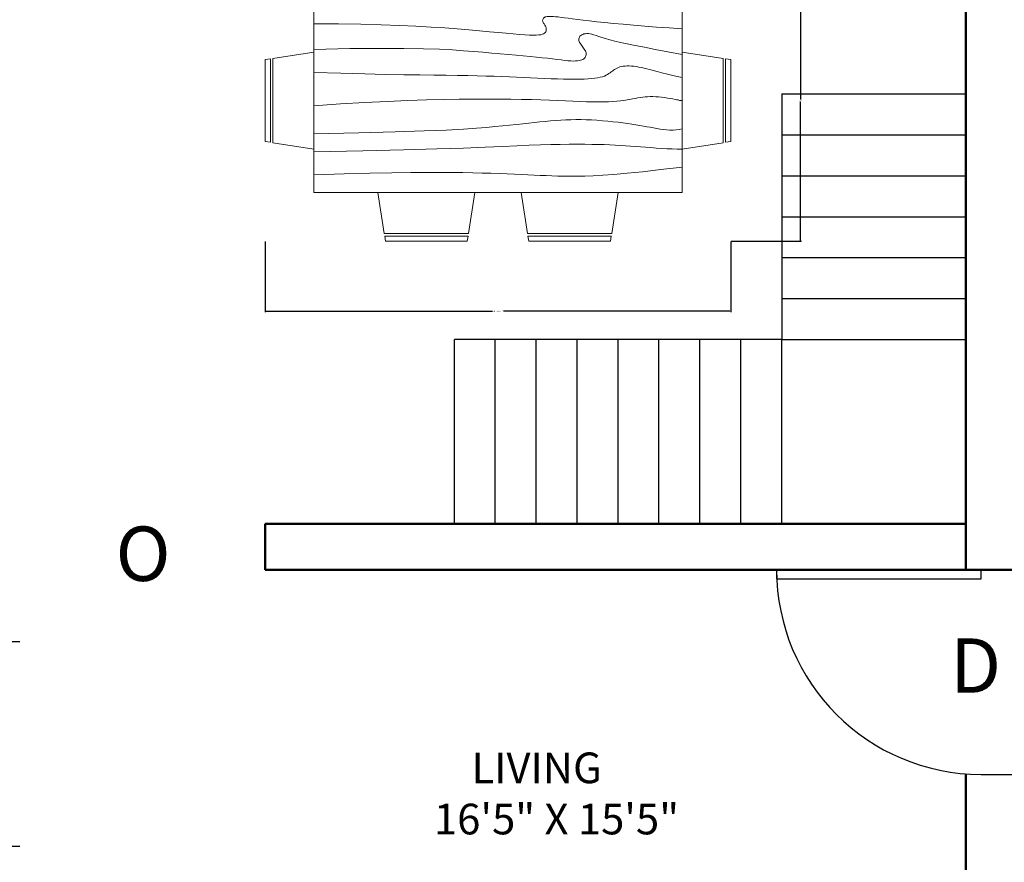
# Model space of a CAD drawing. Units: inches. Extents: x -105 to 1196, y -792 to 119.
# Tile 17 of 23: x 130 to 322, y -285 to -121. Entities that reach past the tile are written whole.
import ezdxf

# ---------------------------------------------------------------- set-up
doc = ezdxf.new("R2010")
doc.units = ezdxf.units.IN
doc.header["$MEASUREMENT"] = 0
for name, color, linetype, lineweight in [('A-ANNO-DIMS', 2, 'Continuous', 18), ('A-ANNO-TEXT', 7, 'Continuous', 25), ('A-AREA-IDEN', 7, 'Continuous', 25), ('A-DOOR', 4, 'Continuous', 25), ('A-FLOR-STRS', 4, 'Continuous', 25), ('A-FURN', 8, 'Continuous', 18), ('A-WALL', 3, 'Continuous', 50)]:
    doc.layers.add(name, color=color, linetype=linetype, lineweight=lineweight)
doc.styles.get("Standard").update_dxf_attribs({"font": 'arial.ttf'})
doc.dimstyles.get("Standard").update_dxf_attribs({"dimtxt": 0.18, "dimasz": 0.18, "dimexe": 0.18, "dimexo": 0.0625, "dimgap": 0.09, "dimtad": 0, "dimtih": 1, "dimtoh": 1, "dimdec": 1, "dimzin": 0, "dimdsep": 46, "dimlunit": 4, "dimtxsty": 'Standard', "dimcen": 0.09, "dimadec": 0, "dimazin": 0, "dimtfac": 1, "dimtdec": 1, "dimtofl": 0, "dimtmove": 0, "dimatfit": 3, "dimfxl": 1, "dimtolj": 1, "dimtzin": 0, "dimarcsym": 0})

# ---------------------------------------------------------------- blocks, each defined once
blk = doc.blocks.new('Dining Set - 36 x 72 in.')
for p, q in [((-22, 27.5), (-22.1562, 26.50042)), ((-22, 27.5), (-6, 27.5)), ((-5.8437, 26.49966), (-6, 27.5)), ((6, 27.5), (5.8438, 26.50042)), ((6, 27.5), (22, 27.5)), ((22.1563, 26.49966), (22, 27.5)), ((-22.2343, 26.00059), (-23.4847, 17.99762)), ((-22.2304, 26), (-5.7608, 26)), ((-5.8416, 26.5), (-22.1534, 26.5)), ((-4.5152, 17.99762), (-5.7655, 25.99926)), ((5.7657, 26.00059), (4.5153, 17.99762)), ((5.7696, 26), (22.2392, 26)), ((22.1584, 26.5), (5.8466, 26.5)), ((23.4848, 17.99762), (22.2345, 25.99926)), ((36, 18), (-36, 18)), ((-36, 18), (-36, -18)), ((36, -18), (36, 18)), ((-45.5, 8), (-44.5004, 8.15617)), ((-45.5, 8), (-45.5, -8)), ((-44.5, -8.15843), (-44.5, 8.15338)), ((-44.0006, 8.23428), (-35.9976, 9.48474)), ((-44, 8.23041), (-44, -8.23915)), ((44.0006, 8.23428), (35.9976, 9.48474)), ((44, 8.23041), (44, -8.23915)), ((44.5, -8.15843), (44.5, 8.15338)), ((45.5, 8), (44.5005, 8.15617)), ((45.5, 8), (45.5, -8)), ((-44.4997, -8.15631), (-45.5, -8)), ((-35.9976, -9.48476), (-43.9993, -8.2345)), ((35.9976, -9.48476), (43.9993, -8.2345)), ((44.4997, -8.15631), (45.5, -8)), ((-36, -18), (36, -18)), ((-22.2343, -26.0006), (-23.4847, -17.99762)), ((-4.5152, -17.99762), (-5.7655, -25.99928)), ((5.7657, -26.0006), (4.5153, -17.99762)), ((23.4848, -17.99762), (22.2345, -25.99928)), ((-22.2304, -26), (-5.7608, -26)), ((-22, -27.5), (-22.1562, -26.50044)), ((-5.8416, -26.5), (-22.1534, -26.5)), ((-5.8437, -26.49967), (-6, -27.5)), ((5.7696, -26), (22.2392, -26)), ((6, -27.5), (5.8438, -26.50044)), ((22.1584, -26.5), (5.8466, -26.5)), ((22.1563, -26.49967), (22, -27.5)), ((-22, -27.5), (-6, -27.5)), ((6, -27.5), (22, -27.5))]:
    blk.add_line(p, q)
for points in [[(-36, 15), (-31.1772, 14.97754), (-26.8079, 14.91406), (-22.8538, 14.81543), (-19.276, 14.6875), (-16.0362, 14.53613), (-13.0957, 14.36718), (-10.4159, 14.18652), (-7.9583, 14), (-5.6904, 13.81315), (-3.6035, 13.63021), (-1.6954, 13.45508), (0.0365, 13.29166), (1.5945, 13.14388), (2.9811, 13.01562), (4.1988, 12.9108), (5.25, 12.83333), (6.1393, 12.78613), (6.8802, 12.76823), (7.4883, 12.77767), (7.9792, 12.8125), (8.3685, 12.87077), (8.6719, 12.95052), (8.9049, 13.0498), (9.0833, 13.16666), (9.2205, 13.29899), (9.3216, 13.44401), (9.3895, 13.59879), (9.4271, 13.76041), (9.4373, 13.92594), (9.4232, 14.09245), (9.3875, 14.257), (9.3333, 14.41666), (9.2638, 14.56917), (9.1836, 14.71484), (9.0975, 14.85465), (9.0104, 14.98958), (8.9272, 15.1206), (8.8529, 15.2487), (8.7922, 15.37483), (8.75, 15.5), (8.7305, 15.62467), (8.7344, 15.74739), (8.7617, 15.86621), (8.8125, 15.97916), (8.8867, 16.08431), (8.9844, 16.17968), (9.1055, 16.26334), (9.25, 16.33333), (9.4189, 16.38802), (9.6172, 16.42708), (9.8506, 16.45052), (10.125, 16.45833), (10.4463, 16.45052), (10.8203, 16.42708), (11.2529, 16.38802), (11.75, 16.33333), (12.3184, 16.26318), (12.9694, 16.17838), (13.7151, 16.07991), (14.5677, 15.96875), (15.5395, 15.84586), (16.6426, 15.71224), (17.8893, 15.56884), (19.2917, 15.41666), (20.859, 15.25667), (22.5879, 15.08984), (24.4721, 14.91715), (26.5052, 14.73958), (28.6809, 14.5581), (30.9929, 14.3737), (33.4347, 14.18733), (36, 14)], [(-36, 10), (-28.9766, 10.14274), (-23.1725, 10.20442), (-18.4241, 10.19775), (-14.5677, 10.13541), (-11.4399, 10.03011), (-8.877, 9.89453), (-6.7154, 9.74137), (-4.7917, 9.58333), (-2.9698, 9.43082), (-1.2246, 9.28515), (0.4415, 9.14534), (2.026, 9.01041), (3.5266, 8.87939), (4.9408, 8.7513), (6.266, 8.62516), (7.5, 8.5), (8.6411, 8.37549), (9.6914, 8.2539), (10.6538, 8.13818), (11.5312, 8.03125), (12.3267, 7.93603), (13.043, 7.85547), (13.6831, 7.79248), (14.25, 7.75), (14.7471, 7.7303), (15.1797, 7.73307), (15.5537, 7.75732), (15.875, 7.80208), (16.1494, 7.86637), (16.3828, 7.94922), (16.5811, 8.04964), (16.75, 8.16666), (16.8944, 8.29915), (17.0143, 8.44531), (17.1089, 8.60319), (17.1771, 8.77083), (17.218, 8.94629), (17.2305, 9.1276), (17.2137, 9.31282), (17.1667, 9.5), (17.0895, 9.6875), (16.987, 9.875), (16.8649, 10.0625), (16.7292, 10.25), (16.5856, 10.4375), (16.4401, 10.625), (16.2985, 10.8125), (16.1667, 11), (16.05, 11.18733), (15.9518, 11.3737), (15.8752, 11.5581), (15.8229, 11.73958), (15.798, 11.91715), (15.8034, 12.08984), (15.842, 12.25667), (15.9167, 12.41666), (16.0295, 12.56836), (16.1784, 12.70833), (16.3605, 12.83268), (16.5729, 12.9375), (16.8127, 13.01888), (17.0768, 13.07291), (17.3625, 13.0957), (17.6667, 13.08333), (17.9894, 13.03312), (18.3418, 12.94726), (18.7382, 12.82918), (19.1927, 12.68229), (19.7195, 12.51001), (20.3327, 12.31575), (21.0465, 12.10294), (21.875, 11.875), (22.8357, 11.63354), (23.959, 11.37304), (25.2786, 11.08618), (26.8282, 10.76562), (28.6414, 10.40405), (30.752, 9.99414), (33.1936, 9.52856), (36, 9)], [(-36, 5.5), (-30.7157, 5.3348), (-26.069, 5.20963), (-21.9946, 5.11767), (-18.4271, 5.05208), (-15.3009, 5.00602), (-12.5508, 4.97265), (-10.1112, 4.94515), (-7.9167, 4.91666), (-5.909, 4.88167), (-4.0586, 4.83984), (-2.3429, 4.79215), (-0.7396, 4.73958), (0.7739, 4.6831), (2.22, 4.6237), (3.6213, 4.56233), (5, 4.5), (6.373, 4.43782), (7.7344, 4.3776), (9.0723, 4.32129), (10.375, 4.27083), (11.6309, 4.22819), (12.8281, 4.19531), (13.9551, 4.17415), (15, 4.16666), (15.954, 4.17448), (16.819, 4.19791), (17.6001, 4.23698), (18.3021, 4.29166), (18.9299, 4.36198), (19.4883, 4.44791), (19.9823, 4.54948), (20.4167, 4.66666), (20.7969, 4.79899), (21.1302, 4.94401), (21.4245, 5.09879), (21.6875, 5.26041), (21.9271, 5.42594), (22.1511, 5.59245), (22.3672, 5.757), (22.5834, 5.91666), (22.8065, 6.06868), (23.0404, 6.21093), (23.2879, 6.34147), (23.5521, 6.45833), (23.8358, 6.55957), (24.142, 6.64323), (24.4735, 6.70735), (24.8334, 6.75), (25.2235, 6.76969), (25.642, 6.76692), (26.0858, 6.74267), (26.5521, 6.69791), (27.0379, 6.63362), (27.5404, 6.55078), (28.0565, 6.45036), (28.5834, 6.33333), (29.1242, 6.19987), (29.7071, 6.04687), (30.3661, 5.87044), (31.1354, 5.66666), (32.0493, 5.43164), (33.142, 5.16146), (34.4475, 4.85221), (36, 4.5)], [(-36, -1), (-30.7915, -0.6591), (-26.0195, -0.38216), (-21.6519, -0.16284), (-17.6563, 0.00521), (-14.0005, 0.12833), (-10.6523, 0.21289), (-7.5796, 0.26522), (-4.75, 0.29166), (-2.134, 0.29793), (0.2878, 0.28711), (2.5317, 0.26163), (4.6146, 0.22396), (6.5529, 0.17651), (8.3633, 0.12174), (10.0623, 0.06209), (11.6667, 0), (13.1899, -0.06201), (14.6341, -0.1211), (15.9982, -0.17432), (17.2813, -0.21875), (18.4823, -0.25147), (19.6003, -0.26953), (20.6343, -0.27002), (21.5834, -0.25), (22.4481, -0.20768), (23.2357, -0.14584), (23.9549, -0.06836), (24.6146, 0.02083), (25.2235, 0.11784), (25.7904, 0.21875), (26.3241, 0.31966), (26.8334, 0.41666), (27.3265, 0.50618), (27.8099, 0.58593), (28.2894, 0.65397), (28.7709, 0.70833), (29.2601, 0.74707), (29.763, 0.76823), (30.2855, 0.76985), (30.8334, 0.75), (31.4088, 0.70784), (31.9994, 0.64713), (32.589, 0.57275), (33.1615, 0.48958), (33.7008, 0.4025), (34.1908, 0.3164), (34.6153, 0.23616), (34.9584, 0.16666), (35.2099, 0.11165), (35.3848, 0.07031), (35.504, 0.04069), (35.5886, 0.02083), (35.6594, 0.00879), (35.7377, 0.0026), (35.8442, 0.00032), (36, 0)], [(-36, -6.5), (-27.1843, -6.31267), (-20.084, -6.1263), (-14.469, -5.9419), (-10.1094, -5.76042), (-6.7752, -5.58285), (-4.2363, -5.41016), (-2.2629, -5.24333), (-0.625, -5.08334), (0.8708, -4.93099), (2.2715, -4.78646), (3.5872, -4.64974), (4.8281, -4.52084), (6.0046, -4.39974), (7.127, -4.28646), (8.2053, -4.18099), (9.25, -4.08334), (10.2705, -3.99382), (11.2734, -3.91407), (12.2647, -3.84603), (13.25, -3.79167), (14.2354, -3.75293), (15.2266, -3.73177), (16.2295, -3.73015), (17.25, -3.75), (18.2912, -3.79248), (19.3451, -3.85547), (20.4009, -3.93604), (21.4479, -4.03125), (22.4754, -4.13819), (23.4727, -4.25391), (24.4289, -4.37549), (25.3334, -4.5), (26.1785, -4.62492), (26.9694, -4.74935), (27.7145, -4.87281), (28.4219, -4.99479), (29.1, -5.11483), (29.7572, -5.23242), (30.4016, -5.34709), (31.0417, -5.45834), (31.6837, -5.56437), (32.3262, -5.65821), (32.9658, -5.73153), (33.599, -5.77604), (34.2224, -5.78345), (34.8327, -5.74545), (35.4264, -5.65373), (36, -5.5)], [(-36, -10), (-26.4022, -9.81299), (-18.4675, -9.62891), (-11.9839, -9.45069), (-6.7396, -9.28125), (-2.5226, -9.12354), (0.8789, -8.98047), (3.6769, -8.85498), (6.0833, -8.75), (8.2767, -8.66765), (10.3021, -8.60677), (12.1712, -8.56543), (13.8958, -8.54167), (15.4876, -8.53353), (16.9583, -8.53907), (18.3197, -8.55632), (19.5834, -8.58334), (20.7616, -8.61841), (21.8685, -8.66081), (22.9188, -8.71004), (23.9271, -8.76563), (24.9081, -8.82707), (25.8763, -8.89388), (26.8465, -8.96558), (27.8334, -9.04167), (28.8474, -9.12118), (29.8828, -9.20117), (30.93, -9.27824), (31.9792, -9.34896), (33.0205, -9.40991), (34.0443, -9.45768), (35.0407, -9.48885), (36, -9.5)], [(-36, -14.5), (-30.0881, -14.33513), (-25.0332, -14.21224), (-20.7312, -14.12647), (-17.0781, -14.07292), (-13.97, -14.04671), (-11.3027, -14.04297), (-8.9724, -14.05681), (-6.875, -14.08334), (-4.9224, -14.11833), (-3.0905, -14.16016), (-1.3709, -14.20785), (0.2448, -14.26042), (1.7647, -14.3169), (3.1973, -14.3763), (4.5507, -14.43767), (5.8333, -14.5), (7.0554, -14.5621), (8.235, -14.62175), (9.3922, -14.67652), (10.5469, -14.72396), (11.7192, -14.76164), (12.929, -14.78711), (14.1965, -14.79794), (15.5417, -14.79167), (16.9933, -14.76424), (18.6152, -14.70508), (20.4804, -14.60197), (22.6615, -14.44271), (25.2312, -14.21509), (28.2624, -13.9069), (31.8277, -13.50594), (36, -13)]]:
    blk.add_lwpolyline(points)
blk = doc.blocks.new('*U24')
for p, q in [((0, 0), (0, -6)), ((-40, 0), (-40, -6))]:
    blk.add_line(p, q)
blk.add_lwpolyline([(0, 0), (0, 40), (-1.75, 40), (-1.75, 0)], close=True)
blk.add_arc((0, 0), 40, 90, 180)
blk = doc.blocks.new('*U4')
for p, q in [((0, 0), (0, -6)), ((40, 0), (40, -6))]:
    blk.add_line(p, q)
blk.add_lwpolyline([(0, 0), (0, 40), (1.75, 40), (1.75, 0)], close=True)
blk.add_arc((0, 0), 40, 0, 90)
blk = doc.blocks.new('*D75')
at = {"layer": 'A-ANNO-DIMS', "color": 0, "lineweight": -2, "transparency": 16777216}
for p, q in [((177.77, -164.1), (177.77, -177.86)), ((268.77, -164.1), (268.77, -177.86)), ((177.95, -177.68), (222.19, -177.68)), ((268.59, -177.68), (224.35, -177.68))]:
    blk.add_line(p, q, dxfattribs=at)
at = {"layer": 'A-ANNO-DIMS', "color": 0, "transparency": 16777216}
for points in [[(177.95, -177.65), (177.95, -177.71), (177.77, -177.68)], [(268.59, -177.65), (268.59, -177.71), (268.77, -177.68)]]:
    blk.add_solid(points, dxfattribs=at)
at = {"layer": 'Defpoints', "color": 0, "transparency": 16777216}
for p in [(177.77, -164.03), (268.77, -164.03), (268.77, -177.68)]:
    blk.add_point(p, dxfattribs=at)
at = {"layer": 'A-ANNO-DIMS', "color": 0, "transparency": 16777216, "insert": (223.27, -177.68), "char_height": 0.18, "attachment_point": 5}
blk.add_mtext('\\A1;DINING SET 7\'-7"', dxfattribs=at)
blk = doc.blocks.new('*D76')
at = {"layer": 'A-ANNO-DIMS', "color": 0, "lineweight": -2, "transparency": 16777216}
for p, q in [((268.83, -109.03), (282.6, -109.03)), ((282.42, -109.21), (282.42, -136.35)), ((282.42, -163.85), (282.42, -136.71)), ((268.83, -164.03), (282.6, -164.03))]:
    blk.add_line(p, q, dxfattribs=at)
at = {"layer": 'A-ANNO-DIMS', "color": 0, "transparency": 16777216}
for points in [[(282.39, -109.21), (282.45, -109.21), (282.42, -109.03)], [(282.39, -163.85), (282.45, -163.85), (282.42, -164.03)]]:
    blk.add_solid(points, dxfattribs=at)
at = {"layer": 'Defpoints', "color": 0, "transparency": 16777216}
for p in [(268.77, -109.03), (282.42, -109.03), (268.77, -164.03)]:
    blk.add_point(p, dxfattribs=at)
at = {"layer": 'A-ANNO-DIMS', "color": 0, "transparency": 16777216, "insert": (282.42, -136.53), "char_height": 0.18, "attachment_point": 5}
blk.add_mtext('\\A1;4\'-7"', dxfattribs=at)

msp = doc.modelspace()

# ---------------------------------------------------------------- linework, layer by layer
at = {"layer": 'A-FLOR-STRS'}
for p, q in [((278.74, -135.23), (314.74, -135.23)), ((278.74, -135.23), (278.74, -183.23)), ((278.74, -143.23), (314.74, -143.23)), ((278.74, -151.23), (314.74, -151.23)), ((278.74, -159.23), (314.74, -159.23)), ((278.74, -167.23), (314.74, -167.23)), ((278.74, -175.23), (314.74, -175.23)), ((214.74, -219.23), (214.74, -183.23)), ((278.74, -183.23), (214.74, -183.23)), ((222.74, -219.23), (222.74, -183.23)), ((230.74, -219.23), (230.74, -183.23)), ((238.74, -219.23), (238.74, -183.23)), ((246.74, -219.23), (246.74, -183.23)), ((254.74, -219.23), (254.74, -183.23)), ((262.74, -219.23), (262.74, -183.23)), ((270.74, -219.23), (270.74, -183.23)), ((278.74, -219.23), (278.74, -183.23)), ((278.74, -183.23), (314.74, -183.23))]:
    msp.add_line(p, q, dxfattribs=at)
at = {"layer": 'A-WALL'}
for p, q in [((314.74, -116.23), (314.74, -228.23)), ((314.74, -219.23), (177.74, -219.23)), ((177.74, -219.23), (177.74, -228.23)), ((323.74, -228.23), (177.74, -228.23)), ((314.74, -268.11), (314.74, -429.23))]:
    msp.add_line(p, q, dxfattribs=at)

# ---------------------------------------------------------------- block references
at = {"layer": 'A-DOOR', "rotation": 90}
for name, p in [('*U24', (317.74, -228.23)), ('*U4', (123.74, -282.23))]:
    msp.add_blockref(name, p, dxfattribs=at)
at = {"layer": 'A-FURN'}
msp.add_blockref('Dining Set - 36 x 72 in.', (223.27, -136.53), dxfattribs=at)

# ---------------------------------------------------------------- texts
at = {"layer": 'A-ANNO-TEXT'}
for s, p in [('O', (148.49, -230.42)), ('D', (311.66, -252.28))]:
    msp.add_text(s, height=10.64, dxfattribs=at).set_placement(p)
at = {"layer": 'A-AREA-IDEN', "insert": (210.74, -263.95), "char_height": 6, "attachment_point": 1}
msp.add_mtext_dynamic_manual_height_columns('    LIVING\\P16\'5" X 15\'5"', width=59.5623, gutter_width=1, heights=[0], dxfattribs=at)

# ---------------------------------------------------------------- dimensions: what is measured, and where the dimension line sits
at = {"layer": 'A-ANNO-DIMS'}
dim = msp.add_linear_dim(base=(282.42, -109.03), p1=(268.77, -164.03), p2=(268.77, -109.03), angle=90, dimstyle='Standard', override={"dimdec": 1, "dimlfac": 1, "dimrnd": 0, "dimzin": 1, "dimdsep": 46, "dimlunit": 4, "dimfrac": 2}, dxfattribs=at)
dim.commit()
dim.dimension.update_dxf_attribs({"geometry": '*D76', "text_midpoint": (282.42, -136.53)})
dim = msp.add_linear_dim(base=(268.77, -177.68), p1=(177.77, -164.03), p2=(268.77, -164.03), text='DINING SET <>', dimstyle='Standard', override={"dimdec": 1, "dimlfac": 1, "dimrnd": 0, "dimzin": 1, "dimdsep": 46, "dimlunit": 4, "dimfrac": 2}, dxfattribs=at)
dim.commit()
dim.dimension.update_dxf_attribs({"geometry": '*D75', "text_midpoint": (223.27, -177.68)})

doc.saveas('drawing.dxf')
